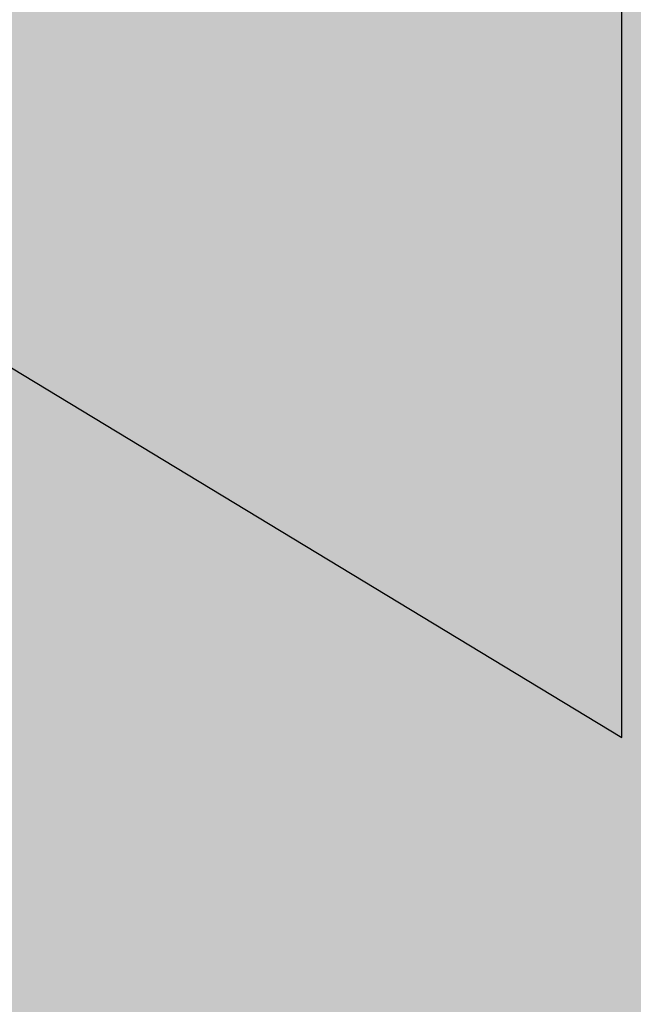
# Model space of a CAD drawing. Units: millimetres. Extents: x -22994 to 29398, y -19990 to 20176.
# Tile 60 of 135: x 223.108 to 225.441, y 79.586 to 83.328. Entities that reach past the tile are written whole.
import ezdxf
from ezdxf import colors
from ezdxf.entities.mleader import LeaderData, LeaderLine
from ezdxf.math import Vec2, Vec3

# ---------------------------------------------------------------- set-up
doc = ezdxf.new("R2010")
doc.units = ezdxf.units.MM
doc.header["$MEASUREMENT"] = 0
for name, color, linetype, lineweight in [('M-ANNO-TEXT', 7, 'Continuous', 25), ('M-DIMS', 2, 'Continuous', 18), ('M-EQPM', 7, 'Continuous', 25), ('M-EQPM-PATT', 7, 'Continuous', 18)]:
    doc.layers.add(name, color=color, linetype=linetype, lineweight=lineweight)
doc.styles.get("Standard").update_dxf_attribs({"font": 'arial.ttf'})
doc.dimstyles.get("Standard").update_dxf_attribs({"dimtxt": 0.18, "dimasz": 10000, "dimexe": 0.18, "dimexo": 0.0625, "dimgap": 0.09, "dimtad": 0, "dimtih": 1, "dimtoh": 1, "dimdec": 0, "dimzin": 0, "dimdsep": 46, "dimtxsty": 'Standard', "dimcen": 0.09, "dimadec": 0, "dimazin": 0, "dimtfac": 1, "dimtdec": 0, "dimtofl": 0, "dimtmove": 0, "dimatfit": 3, "dimfxl": 1, "dimtolj": 1, "dimtzin": 0, "dimlwd": 30, "dimarcsym": 0})

# ---------------------------------------------------------------- blocks, each defined once
blk = doc.blocks.new('*D2')
at = {"layer": 'Defpoints', "color": 0, "transparency": 16777216}
for p in [(6.6773, 10.2713), (290.852, 10.2713), (290.852, -5.0787)]:
    blk.add_point(p, dxfattribs=at)
at = {"layer": 'M-DIMS', "color": 0, "lineweight": -2, "transparency": 16777216}
for p, q in [((6.6773, 10.2088), (6.6773, -5.2587)), ((290.852, 10.2088), (290.852, -5.2587))]:
    blk.add_line(p, q, dxfattribs=at)
at = {"layer": 'M-DIMS', "color": 0, "lineweight": 30, "transparency": 16777216}
for p, q in [((-9993.3227, -5.0787), (-19993.3227, -5.0787)), ((10290.852, -5.0787), (20290.852, -5.0787))]:
    blk.add_line(p, q, dxfattribs=at)
at = {"layer": 'M-DIMS', "color": 0, "transparency": 16777216}
for points in [[(-9993.3227, 1661.5879), (-9993.3227, -1671.7454), (6.6773, -5.0787)], [(10290.852, 1661.5879), (10290.852, -1671.7454), (290.852, -5.0787)]]:
    blk.add_solid(points, dxfattribs=at)
at = {"layer": 'M-DIMS', "color": 0, "transparency": 16777216, "insert": (148.7647, -5.0787), "char_height": 0.18, "attachment_point": 5}
blk.add_mtext('\\A1;284.2', dxfattribs=at)
blk = doc.blocks.new('*D3')
at = {"layer": 'Defpoints', "color": 0, "transparency": 16777216}
for p in [(110.2647, 204.1654), (110.2647, 176.3662), (95.8327, 127.967)]:
    blk.add_point(p, dxfattribs=at)
at = {"layer": 'M-DIMS', "color": 0, "lineweight": -2, "transparency": 16777216}
for p, q in [((95.8327, 128.0295), (95.8327, 204.3454)), ((110.2647, 176.4287), (110.2647, 204.3454))]:
    blk.add_line(p, q, dxfattribs=at)
at = {"layer": 'M-DIMS', "color": 0, "lineweight": 30, "transparency": 16777216}
for p, q in [((-9904.1673, 204.1654), (-19904.1673, 204.1654)), ((10110.2647, 204.1654), (20110.2647, 204.1654))]:
    blk.add_line(p, q, dxfattribs=at)
at = {"layer": 'M-DIMS', "color": 0, "transparency": 16777216}
for points in [[(-9904.1673, 1870.8321), (-9904.1673, -1462.5013), (95.8327, 204.1654)], [(10110.2647, 1870.8321), (10110.2647, -1462.5013), (110.2647, 204.1654)]]:
    blk.add_solid(points, dxfattribs=at)
at = {"layer": 'M-DIMS', "color": 0, "transparency": 16777216, "insert": (103.0487, 204.1654), "char_height": 0.18, "attachment_point": 5}
blk.add_mtext('\\A1;14.432', dxfattribs=at)
blk = doc.blocks.new('*D4')
at = {"layer": 'Defpoints', "color": 0, "transparency": 16777216}
for p in [(116.2647, 204.1654), (110.2647, 176.3662), (116.2647, 176.3662)]:
    blk.add_point(p, dxfattribs=at)
at = {"layer": 'M-DIMS', "color": 0, "lineweight": -2, "transparency": 16777216}
for p, q in [((110.2647, 176.4287), (110.2647, 204.3454)), ((116.2647, 176.4287), (116.2647, 204.3454))]:
    blk.add_line(p, q, dxfattribs=at)
at = {"layer": 'M-DIMS', "color": 0, "lineweight": 30, "transparency": 16777216}
for p, q in [((-9889.7353, 204.1654), (-19889.7353, 204.1654)), ((10116.2647, 204.1654), (20116.2647, 204.1654))]:
    blk.add_line(p, q, dxfattribs=at)
at = {"layer": 'M-DIMS', "color": 0, "transparency": 16777216}
for points in [[(-9889.7353, 1870.8321), (-9889.7353, -1462.5013), (110.2647, 204.1654)], [(10116.2647, 1870.8321), (10116.2647, -1462.5013), (116.2647, 204.1654)]]:
    blk.add_solid(points, dxfattribs=at)
at = {"layer": 'M-DIMS', "color": 0, "transparency": 16777216, "insert": (113.2647, 204.1654), "char_height": 0.18, "attachment_point": 5}
blk.add_mtext('\\A1;6', dxfattribs=at)
blk = doc.blocks.new('*D5')
at = {"layer": 'Defpoints', "color": 0, "transparency": 16777216}
for p in [(181.2647, 204.1654), (116.2647, 176.3662), (181.2647, 176.3662)]:
    blk.add_point(p, dxfattribs=at)
at = {"layer": 'M-DIMS', "color": 0, "lineweight": -2, "transparency": 16777216}
for p, q in [((116.2647, 176.4287), (116.2647, 204.3454)), ((181.2647, 176.4287), (181.2647, 204.3454))]:
    blk.add_line(p, q, dxfattribs=at)
at = {"layer": 'M-DIMS', "color": 0, "lineweight": 30, "transparency": 16777216}
for p, q in [((-9883.7353, 204.1654), (-19883.7353, 204.1654)), ((10181.2647, 204.1654), (20181.2647, 204.1654))]:
    blk.add_line(p, q, dxfattribs=at)
at = {"layer": 'M-DIMS', "color": 0, "transparency": 16777216}
for points in [[(-9883.7353, 1870.8321), (-9883.7353, -1462.5013), (116.2647, 204.1654)], [(10181.2647, 1870.8321), (10181.2647, -1462.5013), (181.2647, 204.1654)]]:
    blk.add_solid(points, dxfattribs=at)
at = {"layer": 'M-DIMS', "color": 0, "transparency": 16777216, "insert": (148.7647, 204.1654), "char_height": 0.18, "attachment_point": 5}
blk.add_mtext('\\A1;65', dxfattribs=at)
blk = doc.blocks.new('*D6')
at = {"layer": 'Defpoints', "color": 0, "transparency": 16777216}
for p in [(187.2647, 204.1654), (181.2647, 176.3662), (187.2647, 176.3662)]:
    blk.add_point(p, dxfattribs=at)
at = {"layer": 'M-DIMS', "color": 0, "lineweight": -2, "transparency": 16777216}
for p, q in [((181.2647, 176.4287), (181.2647, 204.3454)), ((187.2647, 176.4287), (187.2647, 204.3454))]:
    blk.add_line(p, q, dxfattribs=at)
at = {"layer": 'M-DIMS', "color": 0, "lineweight": 30, "transparency": 16777216}
for p, q in [((-9818.7353, 204.1654), (-19818.7353, 204.1654)), ((10187.2647, 204.1654), (20187.2647, 204.1654))]:
    blk.add_line(p, q, dxfattribs=at)
at = {"layer": 'M-DIMS', "color": 0, "transparency": 16777216}
for points in [[(-9818.7353, 1870.8321), (-9818.7353, -1462.5013), (181.2647, 204.1654)], [(10187.2647, 1870.8321), (10187.2647, -1462.5013), (187.2647, 204.1654)]]:
    blk.add_solid(points, dxfattribs=at)
at = {"layer": 'M-DIMS', "color": 0, "transparency": 16777216, "insert": (184.2647, 204.1654), "char_height": 0.18, "attachment_point": 5}
blk.add_mtext('\\A1;6', dxfattribs=at)
blk = doc.blocks.new('*D7')
at = {"layer": 'Defpoints', "color": 0, "transparency": 16777216}
for p in [(201.6967, 204.1654), (187.2647, 176.3662), (201.6967, 127.967)]:
    blk.add_point(p, dxfattribs=at)
at = {"layer": 'M-DIMS', "color": 0, "lineweight": -2, "transparency": 16777216}
for p, q in [((187.2647, 176.4287), (187.2647, 204.3454)), ((201.6967, 128.0295), (201.6967, 204.3454))]:
    blk.add_line(p, q, dxfattribs=at)
at = {"layer": 'M-DIMS', "color": 0, "lineweight": 30, "transparency": 16777216}
for p, q in [((-9812.7353, 204.1654), (-19812.7353, 204.1654)), ((10201.6967, 204.1654), (20201.6967, 204.1654))]:
    blk.add_line(p, q, dxfattribs=at)
at = {"layer": 'M-DIMS', "color": 0, "transparency": 16777216}
for points in [[(-9812.7353, 1870.8321), (-9812.7353, -1462.5013), (187.2647, 204.1654)], [(10201.6967, 1870.8321), (10201.6967, -1462.5013), (201.6967, 204.1654)]]:
    blk.add_solid(points, dxfattribs=at)
at = {"layer": 'M-DIMS', "color": 0, "transparency": 16777216, "insert": (194.4807, 204.1654), "char_height": 0.18, "attachment_point": 5}
blk.add_mtext('\\A1;14.432', dxfattribs=at)
blk = doc.blocks.new('*D8')
at = {"layer": 'Defpoints', "color": 0, "transparency": 16777216}
for p in [(227.6485, 204.1654), (227.6485, 146.7296), (201.6967, 127.967)]:
    blk.add_point(p, dxfattribs=at)
at = {"layer": 'M-DIMS', "color": 0, "lineweight": -2, "transparency": 16777216}
for p, q in [((201.6967, 128.0295), (201.6967, 204.3454)), ((227.6485, 146.7921), (227.6485, 204.3454))]:
    blk.add_line(p, q, dxfattribs=at)
at = {"layer": 'M-DIMS', "color": 0, "lineweight": 30, "transparency": 16777216}
for p, q in [((-9798.3033, 204.1654), (-19798.3033, 204.1654)), ((10227.6485, 204.1654), (20227.6485, 204.1654))]:
    blk.add_line(p, q, dxfattribs=at)
at = {"layer": 'M-DIMS', "color": 0, "transparency": 16777216}
for points in [[(-9798.3033, 1870.8321), (-9798.3033, -1462.5013), (201.6967, 204.1654)], [(10227.6485, 1870.8321), (10227.6485, -1462.5013), (227.6485, 204.1654)]]:
    blk.add_solid(points, dxfattribs=at)
at = {"layer": 'M-DIMS', "color": 0, "transparency": 16777216, "insert": (214.6726, 204.1654), "char_height": 0.18, "attachment_point": 5}
blk.add_mtext('\\A1;25.95', dxfattribs=at)
blk = doc.blocks.new('*D9')
at = {"layer": 'Defpoints', "color": 0, "transparency": 16777216}
for p in [(187.2647, 176.3662), (306.202, 176.3662), (290.852, 10.2713)]:
    blk.add_point(p, dxfattribs=at)
at = {"layer": 'M-DIMS', "color": 0, "lineweight": 30, "transparency": 16777216}
for p, q in [((306.202, 10176.3662), (306.202, 20176.3662)), ((306.202, -9989.7287), (306.202, -19989.7287))]:
    blk.add_line(p, q, dxfattribs=at)
at = {"layer": 'M-DIMS', "color": 0, "lineweight": -2, "transparency": 16777216}
for p, q in [((187.3272, 176.3662), (306.382, 176.3662)), ((290.9145, 10.2713), (306.382, 10.2713))]:
    blk.add_line(p, q, dxfattribs=at)
at = {"layer": 'M-DIMS', "color": 0, "transparency": 16777216}
for points in [[(-1360.4646, 10176.3662), (1972.8687, 10176.3662), (306.202, 176.3662)], [(-1360.4646, -9989.7287), (1972.8687, -9989.7287), (306.202, 10.2713)]]:
    blk.add_solid(points, dxfattribs=at)
at = {"layer": 'M-DIMS', "color": 0, "transparency": 16777216, "insert": (306.202, 93.3187), "char_height": 0.18, "attachment_point": 5}
blk.add_mtext('\\A1;166.1', dxfattribs=at)
blk = doc.blocks.new('*D10')
at = {"layer": 'Defpoints', "color": 0, "transparency": 16777216}
for p in [(125.6498, 136.0713), (133.3459, 136.0713), (133.3459, -5.0787)]:
    blk.add_point(p, dxfattribs=at)
at = {"layer": 'M-DIMS', "color": 0, "lineweight": -2, "transparency": 16777216}
for p, q in [((125.6498, 136.0088), (125.6498, -5.2587)), ((133.3459, 136.0088), (133.3459, -5.2587))]:
    blk.add_line(p, q, dxfattribs=at)
at = {"layer": 'M-DIMS', "color": 0, "lineweight": 30, "transparency": 16777216}
for p, q in [((-9874.3502, -5.0787), (-19874.3502, -5.0787)), ((10133.3459, -5.0787), (20133.3459, -5.0787))]:
    blk.add_line(p, q, dxfattribs=at)
at = {"layer": 'M-DIMS', "color": 0, "transparency": 16777216}
for points in [[(-9874.3502, 1661.5879), (-9874.3502, -1671.7454), (125.6498, -5.0787)], [(10133.3459, 1661.5879), (10133.3459, -1671.7454), (133.3459, -5.0787)]]:
    blk.add_solid(points, dxfattribs=at)
at = {"layer": 'M-DIMS', "color": 0, "transparency": 16777216, "insert": (129.4978, -5.0787), "char_height": 0.18, "attachment_point": 5}
blk.add_mtext('\\A1;7.696', dxfattribs=at)
blk = doc.blocks.new('*D11')
at = {"layer": 'Defpoints', "color": 0, "transparency": 16777216}
for p in [(133.3459, 136.0713), (135.6498, 136.0713), (135.6498, -5.0787)]:
    blk.add_point(p, dxfattribs=at)
at = {"layer": 'M-DIMS', "color": 0, "lineweight": -2, "transparency": 16777216}
for p, q in [((133.3459, 136.0088), (133.3459, -5.2587)), ((135.6498, 136.0088), (135.6498, -5.2587))]:
    blk.add_line(p, q, dxfattribs=at)
at = {"layer": 'M-DIMS', "color": 0, "lineweight": 30, "transparency": 16777216}
for p, q in [((-9866.6541, -5.0787), (-19866.6541, -5.0787)), ((10135.6498, -5.0787), (20135.6498, -5.0787))]:
    blk.add_line(p, q, dxfattribs=at)
at = {"layer": 'M-DIMS', "color": 0, "transparency": 16777216}
for points in [[(-9866.6541, 1661.5879), (-9866.6541, -1671.7454), (133.3459, -5.0787)], [(10135.6498, 1661.5879), (10135.6498, -1671.7454), (135.6498, -5.0787)]]:
    blk.add_solid(points, dxfattribs=at)
at = {"layer": 'M-DIMS', "color": 0, "transparency": 16777216, "insert": (134.4978, -5.0787), "char_height": 0.18, "attachment_point": 5}
blk.add_mtext('\\A1;2.304', dxfattribs=at)
blk = doc.blocks.new('*D12')
at = {"layer": 'Defpoints', "color": 0, "transparency": 16777216}
for p in [(135.6498, 136.0713), (145.6498, 136.0713), (145.6498, -5.0787)]:
    blk.add_point(p, dxfattribs=at)
at = {"layer": 'M-DIMS', "color": 0, "lineweight": -2, "transparency": 16777216}
for p, q in [((135.6498, 136.0088), (135.6498, -5.2587)), ((145.6498, 136.0088), (145.6498, -5.2587))]:
    blk.add_line(p, q, dxfattribs=at)
at = {"layer": 'M-DIMS', "color": 0, "lineweight": 30, "transparency": 16777216}
for p, q in [((-9864.3502, -5.0787), (-19864.3502, -5.0787)), ((10145.6498, -5.0787), (20145.6498, -5.0787))]:
    blk.add_line(p, q, dxfattribs=at)
at = {"layer": 'M-DIMS', "color": 0, "transparency": 16777216}
for points in [[(-9864.3502, 1661.5879), (-9864.3502, -1671.7454), (135.6498, -5.0787)], [(10145.6498, 1661.5879), (10145.6498, -1671.7454), (145.6498, -5.0787)]]:
    blk.add_solid(points, dxfattribs=at)
at = {"layer": 'M-DIMS', "color": 0, "transparency": 16777216, "insert": (140.6498, -5.0787), "char_height": 0.18, "attachment_point": 5}
blk.add_mtext('\\A1;10', dxfattribs=at)
blk = doc.blocks.new('*D13')
at = {"layer": 'Defpoints', "color": 0, "transparency": 16777216}
for p in [(145.6498, 136.0713), (155.6498, 136.0713), (155.6498, -5.0787)]:
    blk.add_point(p, dxfattribs=at)
at = {"layer": 'M-DIMS', "color": 0, "lineweight": -2, "transparency": 16777216}
for p, q in [((145.6498, 136.0088), (145.6498, -5.2587)), ((155.6498, 136.0088), (155.6498, -5.2587))]:
    blk.add_line(p, q, dxfattribs=at)
at = {"layer": 'M-DIMS', "color": 0, "lineweight": 30, "transparency": 16777216}
for p, q in [((-9854.3502, -5.0787), (-19854.3502, -5.0787)), ((10155.6498, -5.0787), (20155.6498, -5.0787))]:
    blk.add_line(p, q, dxfattribs=at)
at = {"layer": 'M-DIMS', "color": 0, "transparency": 16777216}
for points in [[(-9854.3502, 1661.5879), (-9854.3502, -1671.7454), (145.6498, -5.0787)], [(10155.6498, 1661.5879), (10155.6498, -1671.7454), (155.6498, -5.0787)]]:
    blk.add_solid(points, dxfattribs=at)
at = {"layer": 'M-DIMS', "color": 0, "transparency": 16777216, "insert": (150.6498, -5.0787), "char_height": 0.18, "attachment_point": 5}
blk.add_mtext('\\A1;10', dxfattribs=at)
blk = doc.blocks.new('*D14')
at = {"layer": 'Defpoints', "color": 0, "transparency": 16777216}
for p in [(155.6498, 136.0713), (165.6498, 136.0713), (165.6498, -5.0787)]:
    blk.add_point(p, dxfattribs=at)
at = {"layer": 'M-DIMS', "color": 0, "lineweight": -2, "transparency": 16777216}
for p, q in [((155.6498, 136.0088), (155.6498, -5.2587)), ((165.6498, 136.0088), (165.6498, -5.2587))]:
    blk.add_line(p, q, dxfattribs=at)
at = {"layer": 'M-DIMS', "color": 0, "lineweight": 30, "transparency": 16777216}
for p, q in [((-9844.3502, -5.0787), (-19844.3502, -5.0787)), ((10165.6498, -5.0787), (20165.6498, -5.0787))]:
    blk.add_line(p, q, dxfattribs=at)
at = {"layer": 'M-DIMS', "color": 0, "transparency": 16777216}
for points in [[(-9844.3502, 1661.5879), (-9844.3502, -1671.7454), (155.6498, -5.0787)], [(10165.6498, 1661.5879), (10165.6498, -1671.7454), (165.6498, -5.0787)]]:
    blk.add_solid(points, dxfattribs=at)
at = {"layer": 'M-DIMS', "color": 0, "transparency": 16777216, "insert": (160.6498, -5.0787), "char_height": 0.18, "attachment_point": 5}
blk.add_mtext('\\A1;10', dxfattribs=at)
blk = doc.blocks.new('*D15')
at = {"layer": 'Defpoints', "color": 0, "transparency": 16777216}
for p in [(173.3459, 154.788), (173.3459, 136.0713), (306.202, 136.0713)]:
    blk.add_point(p, dxfattribs=at)
at = {"layer": 'M-DIMS', "color": 0, "lineweight": 30, "transparency": 16777216}
for p, q in [((306.202, 10154.788), (306.202, 20154.788)), ((306.202, -9863.9287), (306.202, -19863.9287))]:
    blk.add_line(p, q, dxfattribs=at)
at = {"layer": 'M-DIMS', "color": 0, "lineweight": -2, "transparency": 16777216}
for p, q in [((173.4084, 154.788), (306.382, 154.788)), ((173.4084, 136.0713), (306.382, 136.0713))]:
    blk.add_line(p, q, dxfattribs=at)
at = {"layer": 'M-DIMS', "color": 0, "transparency": 16777216}
for points in [[(-1360.4646, 10154.788), (1972.8687, 10154.788), (306.202, 154.788)], [(-1360.4646, -9863.9287), (1972.8687, -9863.9287), (306.202, 136.0713)]]:
    blk.add_solid(points, dxfattribs=at)
at = {"layer": 'M-DIMS', "color": 0, "transparency": 16777216, "insert": (306.202, 145.4297), "char_height": 0.18, "attachment_point": 5}
blk.add_mtext('\\A1;18.717', dxfattribs=at)
blk = doc.blocks.new('*D16')
at = {"layer": 'Defpoints', "color": 0, "transparency": 16777216}
for p in [(120.1702, 204.1654), (110.4658, 48.0349), (120.1702, 48.0349)]:
    blk.add_point(p, dxfattribs=at)
at = {"layer": 'M-DIMS', "color": 0, "lineweight": -2, "transparency": 16777216}
for p, q in [((110.4658, 48.0974), (110.4658, 204.3454)), ((120.1702, 48.0974), (120.1702, 204.3454))]:
    blk.add_line(p, q, dxfattribs=at)
at = {"layer": 'M-DIMS', "color": 0, "lineweight": 30, "transparency": 16777216}
for p, q in [((-9889.5342, 204.1654), (-19889.5342, 204.1654)), ((10120.1702, 204.1654), (20120.1702, 204.1654))]:
    blk.add_line(p, q, dxfattribs=at)
at = {"layer": 'M-DIMS', "color": 0, "transparency": 16777216}
for points in [[(-9889.5342, 1870.8321), (-9889.5342, -1462.5013), (110.4658, 204.1654)], [(10120.1702, 1870.8321), (10120.1702, -1462.5013), (120.1702, 204.1654)]]:
    blk.add_solid(points, dxfattribs=at)
at = {"layer": 'M-DIMS', "color": 0, "transparency": 16777216, "insert": (115.318, 204.1654), "char_height": 0.18, "attachment_point": 5}
blk.add_mtext('\\A1;9.704', dxfattribs=at)
blk = doc.blocks.new('*D17')
at = {"layer": 'Defpoints', "color": 0, "transparency": 16777216}
for p in [(126.1702, 204.1654), (120.1702, 48.0349), (126.1702, 48.0349)]:
    blk.add_point(p, dxfattribs=at)
at = {"layer": 'M-DIMS', "color": 0, "lineweight": -2, "transparency": 16777216}
for p, q in [((120.1702, 48.0974), (120.1702, 204.3454)), ((126.1702, 48.0974), (126.1702, 204.3454))]:
    blk.add_line(p, q, dxfattribs=at)
at = {"layer": 'M-DIMS', "color": 0, "lineweight": 30, "transparency": 16777216}
for p, q in [((-9879.8298, 204.1654), (-19879.8298, 204.1654)), ((10126.1702, 204.1654), (20126.1702, 204.1654))]:
    blk.add_line(p, q, dxfattribs=at)
at = {"layer": 'M-DIMS', "color": 0, "transparency": 16777216}
for points in [[(-9879.8298, 1870.8321), (-9879.8298, -1462.5013), (120.1702, 204.1654)], [(10126.1702, 1870.8321), (10126.1702, -1462.5013), (126.1702, 204.1654)]]:
    blk.add_solid(points, dxfattribs=at)
at = {"layer": 'M-DIMS', "color": 0, "transparency": 16777216, "insert": (123.1702, 204.1654), "char_height": 0.18, "attachment_point": 5}
blk.add_mtext('\\A1;6', dxfattribs=at)
blk = doc.blocks.new('*D18')
at = {"layer": 'Defpoints', "color": 0, "transparency": 16777216}
for p in [(132.1702, 204.1654), (126.1702, 48.0349), (132.1702, 48.0349)]:
    blk.add_point(p, dxfattribs=at)
at = {"layer": 'M-DIMS', "color": 0, "lineweight": -2, "transparency": 16777216}
for p, q in [((126.1702, 48.0974), (126.1702, 204.3454)), ((132.1702, 48.0974), (132.1702, 204.3454))]:
    blk.add_line(p, q, dxfattribs=at)
at = {"layer": 'M-DIMS', "color": 0, "lineweight": 30, "transparency": 16777216}
for p, q in [((-9873.8298, 204.1654), (-19873.8298, 204.1654)), ((10132.1702, 204.1654), (20132.1702, 204.1654))]:
    blk.add_line(p, q, dxfattribs=at)
at = {"layer": 'M-DIMS', "color": 0, "transparency": 16777216}
for points in [[(-9873.8298, 1870.8321), (-9873.8298, -1462.5013), (126.1702, 204.1654)], [(10132.1702, 1870.8321), (10132.1702, -1462.5013), (132.1702, 204.1654)]]:
    blk.add_solid(points, dxfattribs=at)
at = {"layer": 'M-DIMS', "color": 0, "transparency": 16777216, "insert": (129.1702, 204.1654), "char_height": 0.18, "attachment_point": 5}
blk.add_mtext('\\A1;6', dxfattribs=at)
blk = doc.blocks.new('*D19')
at = {"layer": 'Defpoints', "color": 0, "transparency": 16777216}
for p in [(138.1702, 204.1654), (132.1702, 48.0349), (138.1702, 48.0349)]:
    blk.add_point(p, dxfattribs=at)
at = {"layer": 'M-DIMS', "color": 0, "lineweight": -2, "transparency": 16777216}
for p, q in [((132.1702, 48.0974), (132.1702, 204.3454)), ((138.1702, 48.0974), (138.1702, 204.3454))]:
    blk.add_line(p, q, dxfattribs=at)
at = {"layer": 'M-DIMS', "color": 0, "lineweight": 30, "transparency": 16777216}
for p, q in [((-9867.8298, 204.1654), (-19867.8298, 204.1654)), ((10138.1702, 204.1654), (20138.1702, 204.1654))]:
    blk.add_line(p, q, dxfattribs=at)
at = {"layer": 'M-DIMS', "color": 0, "transparency": 16777216}
for points in [[(-9867.8298, 1870.8321), (-9867.8298, -1462.5013), (132.1702, 204.1654)], [(10138.1702, 1870.8321), (10138.1702, -1462.5013), (138.1702, 204.1654)]]:
    blk.add_solid(points, dxfattribs=at)
at = {"layer": 'M-DIMS', "color": 0, "transparency": 16777216, "insert": (135.1702, 204.1654), "char_height": 0.18, "attachment_point": 5}
blk.add_mtext('\\A1;6', dxfattribs=at)
blk = doc.blocks.new('*D20')
at = {"layer": 'Defpoints', "color": 0, "transparency": 16777216}
for p in [(144.1702, 204.1654), (138.1702, 48.0349), (144.1702, 48.0349)]:
    blk.add_point(p, dxfattribs=at)
at = {"layer": 'M-DIMS', "color": 0, "lineweight": -2, "transparency": 16777216}
for p, q in [((138.1702, 48.0974), (138.1702, 204.3454)), ((144.1702, 48.0974), (144.1702, 204.3454))]:
    blk.add_line(p, q, dxfattribs=at)
at = {"layer": 'M-DIMS', "color": 0, "lineweight": 30, "transparency": 16777216}
for p, q in [((-9861.8298, 204.1654), (-19861.8298, 204.1654)), ((10144.1702, 204.1654), (20144.1702, 204.1654))]:
    blk.add_line(p, q, dxfattribs=at)
at = {"layer": 'M-DIMS', "color": 0, "transparency": 16777216}
for points in [[(-9861.8298, 1870.8321), (-9861.8298, -1462.5013), (138.1702, 204.1654)], [(10144.1702, 1870.8321), (10144.1702, -1462.5013), (144.1702, 204.1654)]]:
    blk.add_solid(points, dxfattribs=at)
at = {"layer": 'M-DIMS', "color": 0, "transparency": 16777216, "insert": (141.1702, 204.1654), "char_height": 0.18, "attachment_point": 5}
blk.add_mtext('\\A1;6', dxfattribs=at)
blk = doc.blocks.new('*D21')
at = {"layer": 'Defpoints', "color": 0, "transparency": 16777216}
for p in [(149.1157, 204.1654), (144.1702, 48.0349), (149.1157, 48.0349)]:
    blk.add_point(p, dxfattribs=at)
at = {"layer": 'M-DIMS', "color": 0, "lineweight": -2, "transparency": 16777216}
for p, q in [((144.1702, 48.0974), (144.1702, 204.3454)), ((149.1157, 48.0974), (149.1157, 204.3454))]:
    blk.add_line(p, q, dxfattribs=at)
at = {"layer": 'M-DIMS', "color": 0, "lineweight": 30, "transparency": 16777216}
for p, q in [((-9855.8298, 204.1654), (-19855.8298, 204.1654)), ((10149.1157, 204.1654), (20149.1157, 204.1654))]:
    blk.add_line(p, q, dxfattribs=at)
at = {"layer": 'M-DIMS', "color": 0, "transparency": 16777216}
for points in [[(-9855.8298, 1870.8321), (-9855.8298, -1462.5013), (144.1702, 204.1654)], [(10149.1157, 1870.8321), (10149.1157, -1462.5013), (149.1157, 204.1654)]]:
    blk.add_solid(points, dxfattribs=at)
at = {"layer": 'M-DIMS', "color": 0, "transparency": 16777216, "insert": (146.6429, 204.1654), "char_height": 0.18, "attachment_point": 5}
blk.add_mtext('\\A1;4.945', dxfattribs=at)
blk = doc.blocks.new('*D22')
at = {"layer": 'Defpoints', "color": 0, "transparency": 16777216}
for p in [(149.1157, 30.9895), (155.1157, 30.9895), (155.1157, -5.0787)]:
    blk.add_point(p, dxfattribs=at)
at = {"layer": 'M-DIMS', "color": 0, "lineweight": -2, "transparency": 16777216}
for p, q in [((149.1157, 30.927), (149.1157, -5.2587)), ((155.1157, 30.927), (155.1157, -5.2587))]:
    blk.add_line(p, q, dxfattribs=at)
at = {"layer": 'M-DIMS', "color": 0, "lineweight": 30, "transparency": 16777216}
for p, q in [((-9850.8843, -5.0787), (-19850.8843, -5.0787)), ((10155.1157, -5.0787), (20155.1157, -5.0787))]:
    blk.add_line(p, q, dxfattribs=at)
at = {"layer": 'M-DIMS', "color": 0, "transparency": 16777216}
for points in [[(-9850.8843, 1661.5879), (-9850.8843, -1671.7454), (149.1157, -5.0787)], [(10155.1157, 1661.5879), (10155.1157, -1671.7454), (155.1157, -5.0787)]]:
    blk.add_solid(points, dxfattribs=at)
at = {"layer": 'M-DIMS', "color": 0, "transparency": 16777216, "insert": (152.1157, -5.0787), "char_height": 0.18, "attachment_point": 5}
blk.add_mtext('\\A1;6', dxfattribs=at)
blk = doc.blocks.new('*D23')
at = {"layer": 'Defpoints', "color": 0, "transparency": 16777216}
for p in [(155.1157, 30.9895), (161.1157, 30.9895), (161.1157, -5.0787)]:
    blk.add_point(p, dxfattribs=at)
at = {"layer": 'M-DIMS', "color": 0, "lineweight": -2, "transparency": 16777216}
for p, q in [((155.1157, 30.927), (155.1157, -5.2587)), ((161.1157, 30.927), (161.1157, -5.2587))]:
    blk.add_line(p, q, dxfattribs=at)
at = {"layer": 'M-DIMS', "color": 0, "lineweight": 30, "transparency": 16777216}
for p, q in [((-9844.8843, -5.0787), (-19844.8843, -5.0787)), ((10161.1157, -5.0787), (20161.1157, -5.0787))]:
    blk.add_line(p, q, dxfattribs=at)
at = {"layer": 'M-DIMS', "color": 0, "transparency": 16777216}
for points in [[(-9844.8843, 1661.5879), (-9844.8843, -1671.7454), (155.1157, -5.0787)], [(10161.1157, 1661.5879), (10161.1157, -1671.7454), (161.1157, -5.0787)]]:
    blk.add_solid(points, dxfattribs=at)
at = {"layer": 'M-DIMS', "color": 0, "transparency": 16777216, "insert": (158.1157, -5.0787), "char_height": 0.18, "attachment_point": 5}
blk.add_mtext('\\A1;6', dxfattribs=at)
blk = doc.blocks.new('*D24')
at = {"layer": 'Defpoints', "color": 0, "transparency": 16777216}
for p in [(161.1157, 30.9895), (166.4387, 30.9895), (166.4387, -5.0787)]:
    blk.add_point(p, dxfattribs=at)
at = {"layer": 'M-DIMS', "color": 0, "lineweight": -2, "transparency": 16777216}
for p, q in [((161.1157, 30.927), (161.1157, -5.2587)), ((166.4387, 30.927), (166.4387, -5.2587))]:
    blk.add_line(p, q, dxfattribs=at)
at = {"layer": 'M-DIMS', "color": 0, "lineweight": 30, "transparency": 16777216}
for p, q in [((-9838.8843, -5.0787), (-19838.8843, -5.0787)), ((10166.4387, -5.0787), (20166.4387, -5.0787))]:
    blk.add_line(p, q, dxfattribs=at)
at = {"layer": 'M-DIMS', "color": 0, "transparency": 16777216}
for points in [[(-9838.8843, 1661.5879), (-9838.8843, -1671.7454), (161.1157, -5.0787)], [(10166.4387, 1661.5879), (10166.4387, -1671.7454), (166.4387, -5.0787)]]:
    blk.add_solid(points, dxfattribs=at)
at = {"layer": 'M-DIMS', "color": 0, "transparency": 16777216, "insert": (163.7772, -5.0787), "char_height": 0.18, "attachment_point": 5}
blk.add_mtext('\\A1;5.323', dxfattribs=at)
blk = doc.blocks.new('*D25')
at = {"layer": 'Defpoints', "color": 0, "transparency": 16777216}
for p in [(166.4387, 30.9895), (172.4387, 30.9895), (172.4387, -5.0787)]:
    blk.add_point(p, dxfattribs=at)
at = {"layer": 'M-DIMS', "color": 0, "lineweight": -2, "transparency": 16777216}
for p, q in [((166.4387, 30.927), (166.4387, -5.2587)), ((172.4387, 30.927), (172.4387, -5.2587))]:
    blk.add_line(p, q, dxfattribs=at)
at = {"layer": 'M-DIMS', "color": 0, "lineweight": 30, "transparency": 16777216}
for p, q in [((-9833.5613, -5.0787), (-19833.5613, -5.0787)), ((10172.4387, -5.0787), (20172.4387, -5.0787))]:
    blk.add_line(p, q, dxfattribs=at)
at = {"layer": 'M-DIMS', "color": 0, "transparency": 16777216}
for points in [[(-9833.5613, 1661.5879), (-9833.5613, -1671.7454), (166.4387, -5.0787)], [(10172.4387, 1661.5879), (10172.4387, -1671.7454), (172.4387, -5.0787)]]:
    blk.add_solid(points, dxfattribs=at)
at = {"layer": 'M-DIMS', "color": 0, "transparency": 16777216, "insert": (169.4387, -5.0787), "char_height": 0.18, "attachment_point": 5}
blk.add_mtext('\\A1;6', dxfattribs=at)
blk = doc.blocks.new('*D26')
at = {"layer": 'Defpoints', "color": 0, "transparency": 16777216}
for p in [(172.4387, 30.9895), (178.4387, 30.9895), (178.4387, -5.0787)]:
    blk.add_point(p, dxfattribs=at)
at = {"layer": 'M-DIMS', "color": 0, "lineweight": -2, "transparency": 16777216}
for p, q in [((172.4387, 30.927), (172.4387, -5.2587)), ((178.4387, 30.927), (178.4387, -5.2587))]:
    blk.add_line(p, q, dxfattribs=at)
at = {"layer": 'M-DIMS', "color": 0, "lineweight": 30, "transparency": 16777216}
for p, q in [((-9827.5613, -5.0787), (-19827.5613, -5.0787)), ((10178.4387, -5.0787), (20178.4387, -5.0787))]:
    blk.add_line(p, q, dxfattribs=at)
at = {"layer": 'M-DIMS', "color": 0, "transparency": 16777216}
for points in [[(-9827.5613, 1661.5879), (-9827.5613, -1671.7454), (172.4387, -5.0787)], [(10178.4387, 1661.5879), (10178.4387, -1671.7454), (178.4387, -5.0787)]]:
    blk.add_solid(points, dxfattribs=at)
at = {"layer": 'M-DIMS', "color": 0, "transparency": 16777216, "insert": (175.4387, -5.0787), "char_height": 0.18, "attachment_point": 5}
blk.add_mtext('\\A1;6', dxfattribs=at)
blk = doc.blocks.new('*D27')
at = {"layer": 'Defpoints', "color": 0, "transparency": 16777216}
for p in [(178.4387, 30.9895), (188.1175, 30.9895), (188.1175, -5.0787)]:
    blk.add_point(p, dxfattribs=at)
at = {"layer": 'M-DIMS', "color": 0, "lineweight": -2, "transparency": 16777216}
for p, q in [((178.4387, 30.927), (178.4387, -5.2587)), ((188.1175, 30.927), (188.1175, -5.2587))]:
    blk.add_line(p, q, dxfattribs=at)
at = {"layer": 'M-DIMS', "color": 0, "lineweight": 30, "transparency": 16777216}
for p, q in [((-9821.5613, -5.0787), (-19821.5613, -5.0787)), ((10188.1175, -5.0787), (20188.1175, -5.0787))]:
    blk.add_line(p, q, dxfattribs=at)
at = {"layer": 'M-DIMS', "color": 0, "transparency": 16777216}
for points in [[(-9821.5613, 1661.5879), (-9821.5613, -1671.7454), (178.4387, -5.0787)], [(10188.1175, 1661.5879), (10188.1175, -1671.7454), (188.1175, -5.0787)]]:
    blk.add_solid(points, dxfattribs=at)
at = {"layer": 'M-DIMS', "color": 0, "transparency": 16777216, "insert": (183.2781, -5.0787), "char_height": 0.18, "attachment_point": 5}
blk.add_mtext('\\A1;9.679', dxfattribs=at)
blk = doc.blocks.new('*D28')
at = {"layer": 'Defpoints', "color": 0, "transparency": 16777216}
for p in [(188.1175, 48.0349), (306.202, 48.0349), (188.1175, 30.9895)]:
    blk.add_point(p, dxfattribs=at)
at = {"layer": 'M-DIMS', "color": 0, "lineweight": 30, "transparency": 16777216}
for p, q in [((306.202, 10048.0349), (306.202, 20048.0349)), ((306.202, -9969.0105), (306.202, -19969.0105))]:
    blk.add_line(p, q, dxfattribs=at)
at = {"layer": 'M-DIMS', "color": 0, "lineweight": -2, "transparency": 16777216}
for p, q in [((188.18, 48.0349), (306.382, 48.0349)), ((188.18, 30.9895), (306.382, 30.9895))]:
    blk.add_line(p, q, dxfattribs=at)
at = {"layer": 'M-DIMS', "color": 0, "transparency": 16777216}
for points in [[(-1360.4646, 10048.0349), (1972.8687, 10048.0349), (306.202, 48.0349)], [(-1360.4646, -9969.0105), (1972.8687, -9969.0105), (306.202, 30.9895)]]:
    blk.add_solid(points, dxfattribs=at)
at = {"layer": 'M-DIMS', "color": 0, "transparency": 16777216, "insert": (306.202, 39.5122), "char_height": 0.18, "attachment_point": 5}
blk.add_mtext('\\A1;17.045', dxfattribs=at)
blk = doc.blocks.new('*D29')
at = {"layer": 'Defpoints', "color": 0, "transparency": 16777216}
for p in [(36.8006, 80.045), (64.0296, 80.045)]:
    blk.add_point(p, dxfattribs=at)
at = {"layer": 'M-DIMS', "color": 0, "lineweight": -2, "transparency": 16777216}
for p, q in [((50.4151, 79.955), (50.4151, 80.135)), ((50.3251, 80.045), (50.5051, 80.045))]:
    blk.add_line(p, q, dxfattribs=at)
at = {"layer": 'M-DIMS', "color": 0, "lineweight": 30, "transparency": 16777216}
blk.add_line((20064.0296, 80.0303), (10064.0296, 80.0377), dxfattribs=at)
at = {"layer": 'M-DIMS', "color": 0, "transparency": 16777216}
blk.add_solid([(10064.0309, 1746.7043), (10064.0284, -1586.629), (64.0296, 80.045)], dxfattribs=at)
at = {"layer": 'M-DIMS', "color": 0, "transparency": 16777216, "insert": (20064.5213, 80.0303), "char_height": 0.18, "attachment_point": 5}
blk.add_mtext('\\A1;∅27.23', dxfattribs=at)
blk = doc.blocks.new('*D30')
at = {"layer": 'Defpoints', "color": 0, "transparency": 16777216}
for p in [(216.3148, 146.7291), (238.9821, 146.73)]:
    blk.add_point(p, dxfattribs=at)
at = {"layer": 'M-DIMS', "color": 0, "lineweight": 30, "transparency": 16777216}
blk.add_line((20238.9821, 147.4959), (10238.9821, 147.1129), dxfattribs=at)
at = {"layer": 'M-DIMS', "color": 0, "lineweight": -2, "transparency": 16777216}
for p, q in [((227.6485, 146.6396), (227.6485, 146.8196)), ((227.5585, 146.7296), (227.7385, 146.7296))]:
    blk.add_line(p, q, dxfattribs=at)
at = {"layer": 'M-DIMS', "color": 0, "transparency": 16777216}
blk.add_solid([(10238.9183, 1813.7796), (10239.0459, -1519.5537), (238.9821, 146.73)], dxfattribs=at)
at = {"layer": 'M-DIMS', "color": 0, "transparency": 16777216, "insert": (20239.5436, 147.4959), "char_height": 0.18, "attachment_point": 5}
blk.add_mtext('\\A1;∅22.667', dxfattribs=at)
blk = doc.blocks.new('*D31')
at = {"layer": 'Defpoints', "color": 0, "transparency": 16777216}
for p in [(223.1641, 146.7291), (232.1328, 146.73)]:
    blk.add_point(p, dxfattribs=at)
at = {"layer": 'M-DIMS', "color": 0, "lineweight": 30, "transparency": 16777216}
blk.add_line((20232.1327, 148.6656), (10232.1328, 147.6978), dxfattribs=at)
at = {"layer": 'M-DIMS', "color": 0, "lineweight": -2, "transparency": 16777216}
for p, q in [((227.6485, 146.6396), (227.6485, 146.8196)), ((227.5585, 146.7296), (227.7385, 146.7296))]:
    blk.add_line(p, q, dxfattribs=at)
at = {"layer": 'M-DIMS', "color": 0, "transparency": 16777216}
blk.add_solid([(10231.9715, 1814.3645), (10232.2941, -1518.9688), (232.1328, 146.73)], dxfattribs=at)
at = {"layer": 'M-DIMS', "color": 0, "transparency": 16777216, "insert": (20232.6245, 148.6656), "char_height": 0.18, "attachment_point": 5}
blk.add_mtext('\\A1;∅8.969', dxfattribs=at)
blk = doc.blocks.new('*D36')
at = {"layer": 'Defpoints', "color": 0, "transparency": 16777216}
for p in [(46.39, 31.3035), (46.3875, 26.5934)]:
    blk.add_point(p, dxfattribs=at)
at = {"layer": 'M-DIMS', "color": 0, "lineweight": 30, "transparency": 16777216}
for p, q in [((57.1499, 20031.3006), (51.77, 10031.302)), ((10057.1499, 20031.3006), (57.1499, 20031.3006))]:
    blk.add_line(p, q, dxfattribs=at)
at = {"layer": 'M-DIMS', "color": 0, "lineweight": -2, "transparency": 16777216}
for p, q in [((46.3887, 28.8585), (46.3887, 29.0385)), ((46.2987, 28.9485), (46.4787, 28.9485))]:
    blk.add_line(p, q, dxfattribs=at)
at = {"layer": 'M-DIMS', "color": 0, "transparency": 16777216}
blk.add_solid([(-1614.8965, 10032.1987), (1718.4364, 10030.4054), (46.39, 31.3035)], dxfattribs=at)
at = {"layer": 'M-DIMS', "color": 0, "transparency": 16777216, "insert": (10057.5542, 20031.3006), "char_height": 0.18, "attachment_point": 5}
blk.add_mtext('\\A1;∅4.71', dxfattribs=at)

msp = doc.modelspace()

# ---------------------------------------------------------------- hatches: boundary and pattern name
at = {"layer": 'M-EQPM-PATT'}
h = msp.add_hatch(color=256, dxfattribs=at)
h.set_gradient(color1=(205, 32, 39), color2=(205, 32, 39), tint=1)
h.paths.add_polyline_path([(116.2647, 150.3662), (116.2647, 170.3662), (116.2647, 176.3662), (110.2647, 176.3662), (110.2647, 152.0276), (95.8327, 127.967), (95.8327, 16.6063), (201.6967, 16.6063), (201.6967, 127.967), (187.2647, 152.0276), (187.2647, 176.3662), (181.2647, 176.3662), (181.2647, 170.3662), (181.2647, 150.3662), (195.6967, 126.3055), (195.6967, 22.6063), (101.8327, 22.6063), (101.8327, 126.3055)])
h.paths.add_polyline_path([(185.2208, 88.6347), (101.8327, 88.6347), (101.8327, 87.6347), (182.8066, 87.6347), (178.7313, 83.5594), (195.6967, 83.5594), (195.6967, 84.5594), (181.1455, 84.5594)], flags=17)
h.paths.add_polyline_path([(95.8327, 88.6347), (60.9779, 88.6347, -0.022855), (61.7178, 87.6347), (95.8327, 87.6347)])
h.paths.add_polyline_path([(215.6212, 86.5189), (215.6212, 80.5999), (220.5095, 83.5594)])
h.paths.add_polyline_path([(215.6212, 84.5594), (201.6967, 84.5594), (201.6967, 83.5594), (215.6212, 83.5594)])
h.paths.add_polyline_path([(225.3978, 86.5189), (220.5095, 83.5594), (225.3978, 80.5999)])
h.paths.add_polyline_path([(231.6256, 84.5594), (225.3978, 84.5594), (225.3978, 83.5594), (231.6256, 83.5594)])

# ---------------------------------------------------------------- linework, layer by layer
at = {"layer": 'M-EQPM'}
msp.add_lwpolyline([(225.3978, 86.5189), (215.6212, 80.5999), (215.6212, 86.5189), (225.3978, 80.5999)], close=True, dxfattribs=at)

# ---------------------------------------------------------------- dimensions: what is measured, and where the dimension line sits
at = {"layer": 'M-DIMS'}
for base, p1, p2, override, picture, middle in [((306.202, 176.3662), (290.852, 10.2713), (187.2647, 176.3662), {"dimdec": 1, "dimlfac": 1, "dimrnd": 0, "dimzin": 0, "dimdsep": 46, "dimlunit": 2}, '*D9', (306.202, 93.3187)), ((306.202, 136.0713), (173.3459, 154.788), (173.3459, 136.0713), {"dimdec": 3, "dimlfac": 1, "dimrnd": 0, "dimzin": 0, "dimdsep": 46, "dimlunit": 2}, '*D15', (306.202, 145.4297)), ((306.202, 48.0349), (188.1175, 30.9895), (188.1175, 48.0349), {"dimdec": 3, "dimlfac": 1, "dimrnd": 0, "dimzin": 0, "dimdsep": 46, "dimlunit": 2}, '*D28', (306.202, 39.5122))]:
    dim = msp.add_linear_dim(base=base, p1=p1, p2=p2, angle=90, dimstyle='Standard', override=override, dxfattribs=at)
    dim.commit()
    dim.dimension.update_dxf_attribs({"geometry": picture, "text_midpoint": middle})
for p1, p2, override, picture, middle in [((46.3875, 26.5934), (46.39, 31.3035), {"dimdec": 2, "dimlfac": 1, "dimrnd": 0, "dimzin": 0, "dimdsep": 46, "dimlunit": 2}, '*D36', (10057.5542, 20031.3006)), ((223.1641, 146.7291), (232.1328, 146.73), {"dimdec": 3, "dimlfac": 1, "dimrnd": 0, "dimzin": 0, "dimdsep": 46, "dimlunit": 2}, '*D31', (20232.1327, 148.6656)), ((216.3148, 146.7291), (238.9821, 146.73), {"dimdec": 3, "dimlfac": 1, "dimrnd": 0, "dimzin": 0, "dimdsep": 46, "dimlunit": 2}, '*D30', (20238.9821, 147.4959))]:
    dim = msp.add_diameter_dim_2p(p1=p1, p2=p2, dimstyle='Standard', override=override, dxfattribs=at)
    dim.commit()
    dim.dimension.update_dxf_attribs({"geometry": picture, "text_midpoint": middle, "dimtype": 163})
for base, p1, p2, override, picture, middle in [((110.2647, 204.1654), (95.8327, 127.967), (110.2647, 176.3662), {"dimdec": 3, "dimlfac": 1, "dimrnd": 0, "dimzin": 0, "dimdsep": 46, "dimlunit": 2}, '*D3', (103.0487, 204.1654)), ((116.2647, 204.1654), (110.2647, 176.3662), (116.2647, 176.3662), {"dimdec": 0, "dimlfac": 1, "dimrnd": 0, "dimzin": 0, "dimdsep": 46, "dimlunit": 2}, '*D4', (113.2647, 204.1654)), ((120.1702, 204.1654), (110.4658, 48.0349), (120.1702, 48.0349), {"dimdec": 3, "dimlfac": 1, "dimrnd": 0, "dimzin": 0, "dimdsep": 46, "dimlunit": 2}, '*D16', (115.318, 204.1654)), ((181.2647, 204.1654), (116.2647, 176.3662), (181.2647, 176.3662), {"dimdec": 0, "dimlfac": 1, "dimrnd": 0, "dimzin": 0, "dimdsep": 46, "dimlunit": 2}, '*D5', (148.7647, 204.1654)), ((126.1702, 204.1654), (120.1702, 48.0349), (126.1702, 48.0349), {"dimdec": 0, "dimlfac": 1, "dimrnd": 0, "dimzin": 0, "dimdsep": 46, "dimlunit": 2}, '*D17', (123.1702, 204.1654)), ((132.1702, 204.1654), (126.1702, 48.0349), (132.1702, 48.0349), {"dimdec": 0, "dimlfac": 1, "dimrnd": 0, "dimzin": 0, "dimdsep": 46, "dimlunit": 2}, '*D18', (129.1702, 204.1654)), ((138.1702, 204.1654), (132.1702, 48.0349), (138.1702, 48.0349), {"dimdec": 0, "dimlfac": 1, "dimrnd": 0, "dimzin": 0, "dimdsep": 46, "dimlunit": 2}, '*D19', (135.1702, 204.1654)), ((144.1702, 204.1654), (138.1702, 48.0349), (144.1702, 48.0349), {"dimdec": 0, "dimlfac": 1, "dimrnd": 0, "dimzin": 0, "dimdsep": 46, "dimlunit": 2}, '*D20', (141.1702, 204.1654)), ((149.11567, 204.16539), (144.17023, 48.03494), (149.11567, 48.03494), {"dimdec": 3, "dimlfac": 1, "dimrnd": 0, "dimzin": 0, "dimdsep": 46, "dimlunit": 2}, '*D21', (146.64295, 204.16539)), ((187.2647, 204.1654), (181.2647, 176.3662), (187.2647, 176.3662), {"dimdec": 0, "dimlfac": 1, "dimrnd": 0, "dimzin": 0, "dimdsep": 46, "dimlunit": 2}, '*D6', (184.2647, 204.1654)), ((201.6967, 204.1654), (187.2647, 176.3662), (201.6967, 127.967), {"dimdec": 3, "dimlfac": 1, "dimrnd": 0, "dimzin": 0, "dimdsep": 46, "dimlunit": 2}, '*D7', (194.4807, 204.1654)), ((227.6485, 204.1654), (201.6967, 127.967), (227.6485, 146.7296), {"dimdec": 2, "dimlfac": 1, "dimrnd": 0, "dimzin": 0, "dimdsep": 46, "dimlunit": 2}, '*D8', (214.6726, 204.1654)), ((290.852, -5.0787), (6.6773, 10.2713), (290.852, 10.2713), {"dimdec": 1, "dimlfac": 1, "dimrnd": 0, "dimzin": 0, "dimdsep": 46, "dimlunit": 2}, '*D2', (148.7647, -5.0787)), ((133.3459, -5.0787), (125.6498, 136.0713), (133.3459, 136.0713), {"dimdec": 3, "dimlfac": 1, "dimrnd": 0, "dimzin": 0, "dimdsep": 46, "dimlunit": 2}, '*D10', (129.4978, -5.0787)), ((135.6498, -5.0787), (133.3459, 136.0713), (135.6498, 136.0713), {"dimdec": 3, "dimlfac": 1, "dimrnd": 0, "dimzin": 0, "dimdsep": 46, "dimlunit": 2}, '*D11', (134.4978, -5.0787)), ((145.6498, -5.0787), (135.6498, 136.0713), (145.6498, 136.0713), {"dimdec": 0, "dimlfac": 1, "dimrnd": 0, "dimzin": 0, "dimdsep": 46, "dimlunit": 2}, '*D12', (140.6498, -5.0787)), ((155.6498, -5.0787), (145.6498, 136.0713), (155.6498, 136.0713), {"dimdec": 0, "dimlfac": 1, "dimrnd": 0, "dimzin": 0, "dimdsep": 46, "dimlunit": 2}, '*D13', (150.6498, -5.0787)), ((155.1157, -5.0787), (149.1157, 30.9895), (155.1157, 30.9895), {"dimdec": 0, "dimlfac": 1, "dimrnd": 0, "dimzin": 0, "dimdsep": 46, "dimlunit": 2}, '*D22', (152.1157, -5.0787)), ((161.1157, -5.0787), (155.1157, 30.9895), (161.1157, 30.9895), {"dimdec": 0, "dimlfac": 1, "dimrnd": 0, "dimzin": 0, "dimdsep": 46, "dimlunit": 2}, '*D23', (158.1157, -5.0787)), ((165.6498, -5.0787), (155.6498, 136.0713), (165.6498, 136.0713), {"dimdec": 0, "dimlfac": 1, "dimrnd": 0, "dimzin": 0, "dimdsep": 46, "dimlunit": 2}, '*D14', (160.6498, -5.0787)), ((166.4387, -5.0787), (161.1157, 30.9895), (166.4387, 30.9895), {"dimdec": 3, "dimlfac": 1, "dimrnd": 0, "dimzin": 0, "dimdsep": 46, "dimlunit": 2}, '*D24', (163.7772, -5.0787)), ((172.4387, -5.0787), (166.4387, 30.9895), (172.4387, 30.9895), {"dimdec": 0, "dimlfac": 1, "dimrnd": 0, "dimzin": 0, "dimdsep": 46, "dimlunit": 2}, '*D25', (169.4387, -5.0787)), ((178.4387, -5.0787), (172.4387, 30.9895), (178.4387, 30.9895), {"dimdec": 0, "dimlfac": 1, "dimrnd": 0, "dimzin": 0, "dimdsep": 46, "dimlunit": 2}, '*D26', (175.4387, -5.0787)), ((188.1175, -5.0787), (178.4387, 30.9895), (188.1175, 30.9895), {"dimdec": 3, "dimlfac": 1, "dimrnd": 0, "dimzin": 0, "dimdsep": 46, "dimlunit": 2}, '*D27', (183.2781, -5.0787))]:
    dim = msp.add_linear_dim(base=base, p1=p1, p2=p2, dimstyle='Standard', override=override, dxfattribs=at)
    dim.commit()
    dim.dimension.update_dxf_attribs({"geometry": picture, "text_midpoint": middle})
dim = msp.add_diameter_dim_2p(p1=(36.8006, 80.045), p2=(64.0296, 80.045), dimstyle='Standard', override={"dimdec": 2, "dimlfac": 1, "dimrnd": 0, "dimzin": 0, "dimdsep": 46, "dimlunit": 2}, dxfattribs=at)
dim.commit()
dim.dimension.update_dxf_attribs({"geometry": '*D29', "text_midpoint": (20064.0296, 80.0303)})

# ---------------------------------------------------------------- leaders
at = {"layer": 'M-ANNO-TEXT'}
ml = msp.add_multileader_mtext('Standard', dxfattribs=at)
ml.set_content('combustion chamber', color=256)
ml.set_leader_properties()
ml.build(insert=Vec2(0, 0))
ml.multileader.update_dxf_attribs({"dogleg_length": 0.36, "arrow_head_size": 200})
ctx = ml.context
ctx.base_point, ctx.char_height, ctx.arrow_head_size, ctx.landing_gap_size, ctx.plane_origin = Vec3(215.7321, 57.9149), 3, 200, 0.09, Vec3(189.1175, 57.9149)
notes = []
notes.append((ctx, [(0, (1, 1, 0), (215.3721, 57.9149), (1, 0), 0.36, [(0, [(189.1175, 57.9149)], 0, [])])]))
ctx.mtext.insert, ctx.mtext.flow_direction = Vec3(215.8221, 59.4394), 5
for ctx, leaders in notes:
    for number, flags, end, landing, length, lines in leaders:
        leader = LeaderData()
        leader.index, (leader.has_last_leader_line, leader.has_dogleg_vector, leader.attachment_direction) = number, flags
        leader.last_leader_point, leader.dogleg_vector, leader.dogleg_length = Vec3(end), Vec3(landing), length
        for number, points, colour, breaks in lines:
            line = LeaderLine()
            line.index, line.vertices, line.color, line.breaks = number, Vec3.list(points), colors.encode_raw_color(colour), breaks
            leader.lines.append(line)
        ctx.leaders.append(leader)

doc.saveas('drawing.dxf')
